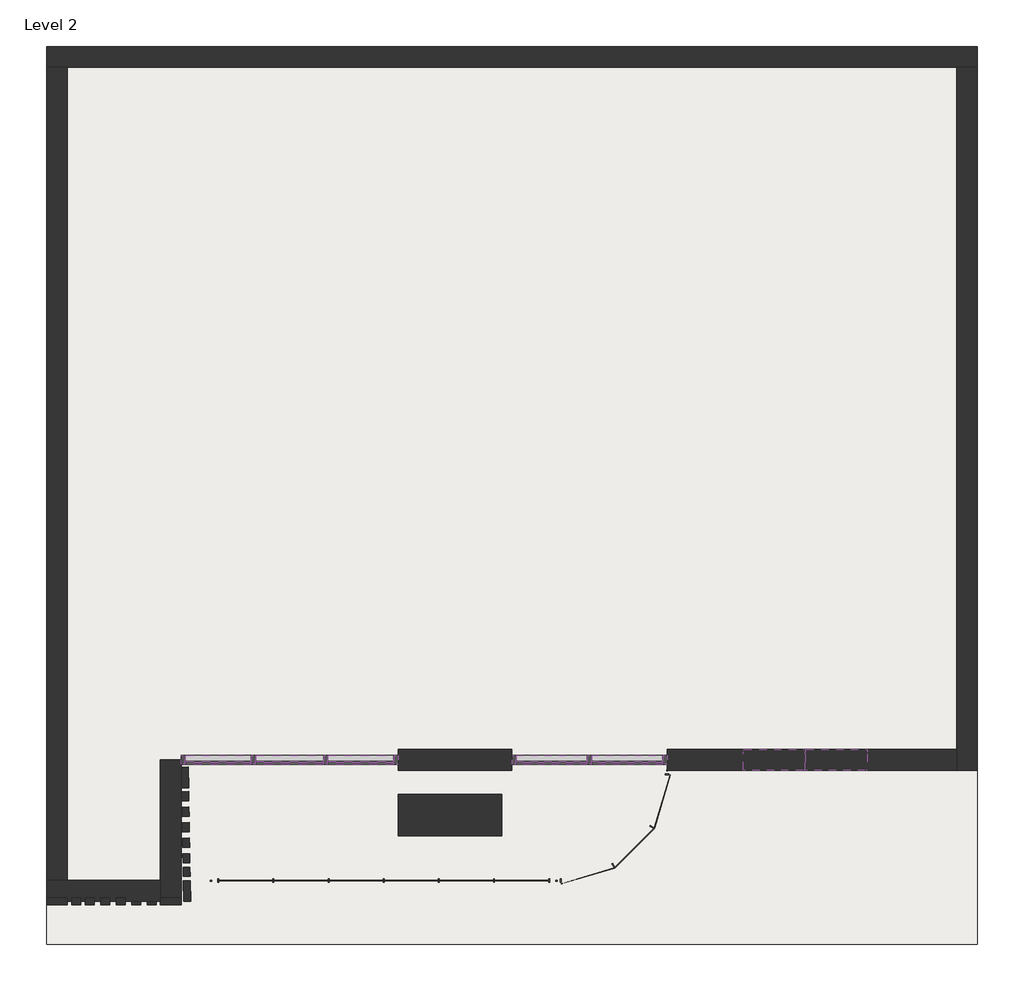
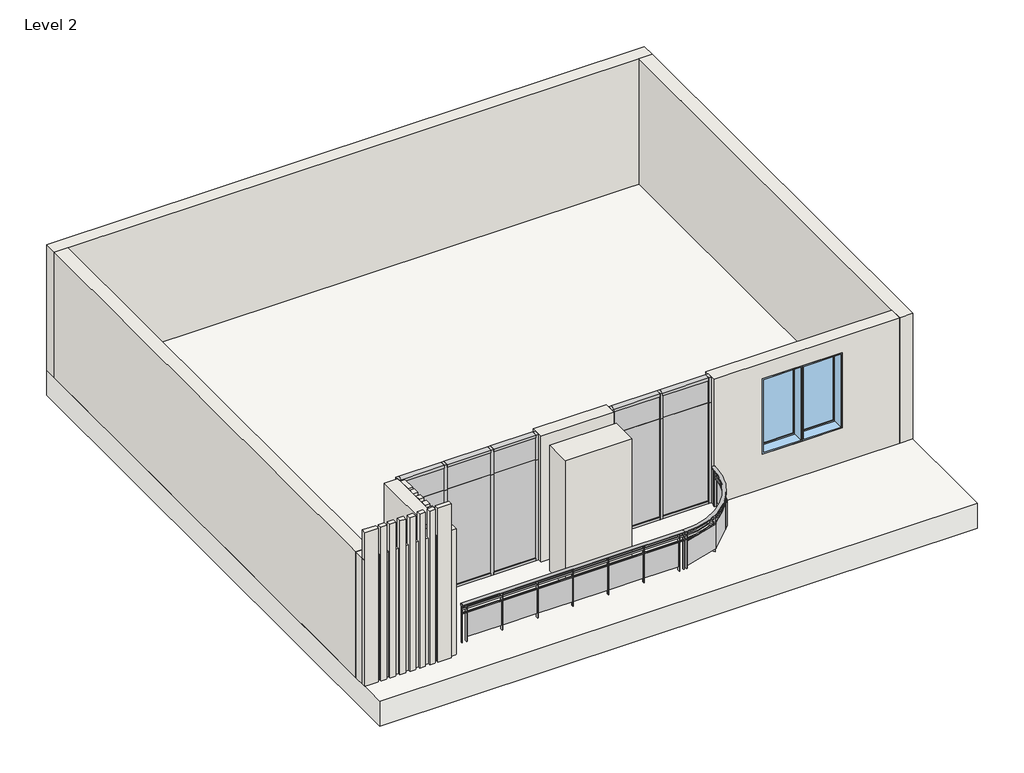
# One storey: 24 members, 24 walls, 10 plates, 2 windows, 1 railing, 1 roof.
"""IFC4 building model written with IfcOpenShell, lengths in millimetres."""

from ifc_helpers import new_model, si_unit, point, frame, origin, place, context, project, spatial, polyline, circle_curve, ellipse_curve, trimmed, outline, extrude, faceted_brep, transform, mapped, element, save
from ifc_brep_helpers import plane_surface, cylinder_surface, revolved_surface, extruded_surface, advanced_brep
from components import member_78934672, member_801a2072, member_cfcad22e, member_ee409385, member_47bfaf8a, member_f0fea5a5, member_6e77e263, system_panel_glazed_66ef8e2c, system_panel_glazed_30b75583, system_panel_glazed_387c9df4, system_panel_glazed_55a8196a, system_panel_glazed_9df4f396, system_panel_glazed_c1629c18, window_9a1f8bc2, window_c524ad49

model = new_model("IFC4")

# Units and contexts
model_context = context("Model", 3, world=origin())
ifc_project = project(units=[si_unit("LENGTHUNIT", "METRE", prefix="MILLI")], contexts=[model_context])

# Site, building, storey
site = spatial("IfcSite", under=ifc_project)
building = spatial("IfcBuilding", under=site)
storey = spatial("IfcBuildingStorey", under=building, Name="Level 2", Elevation=3048.0)

# Members
placement = place(None, origin())
member_shape = member_78934672(model_context)
element("IfcMember", 1, ObjectType="Rectangular Mullion : 2.5\" x 5\" rectangular", at=placement, inside=storey, context=model_context, shape_type="MappedRepresentation", body=[
    mapped(member_shape, transform((-10103.7104559, 977.728737, 3657.6), x_axis=(0.0, 0.0, -1.0), y_axis=(0.0, 1.0, 0.0), z_axis=(1.0, 0.0, 0.0))),
])
element("IfcMember", 2, ObjectType="Rectangular Mullion : 2.5\" x 5\" rectangular", at=placement, inside=storey, context=model_context, shape_type="MappedRepresentation", body=[
    mapped(member_shape, transform((-11214.9604559, 977.728737, 3657.6), x_axis=(0.0, 0.0, -1.0), y_axis=(0.0, 1.0, 0.0), z_axis=(1.0, 0.0, 0.0))),
])
element("IfcMember", 3, ObjectType="Rectangular Mullion : 2.5\" x 5\" rectangular", at=placement, inside=storey, context=model_context, shape_type="MappedRepresentation", body=[
    mapped(member_shape, transform((-12262.7104559, 977.728737, 6705.6), x_axis=(0.0, 0.0, 1.0), y_axis=(0.0, 1.0, 0.0), z_axis=(-1.0, 0.0, 0.0))),
])
element("IfcMember", 4, ObjectType="Rectangular Mullion : 2.5\" x 5\" rectangular", at=placement, inside=storey, context=model_context, shape_type="MappedRepresentation", body=[
    mapped(member_shape, transform((-11151.4604559, 977.728737, 6705.6), x_axis=(0.0, 0.0, 1.0), y_axis=(0.0, 1.0, 0.0), z_axis=(-1.0, 0.0, 0.0))),
])
member_2_shape = member_801a2072(model_context)
element("IfcMember", 5, ObjectType="Rectangular Mullion : 2.5\" x 5\" rectangular", at=placement, inside=storey, context=model_context, shape_type="MappedRepresentation", body=[
    mapped(member_2_shape, transform((-17139.5104559, 977.728737, 6705.6), x_axis=(0.0, 0.0, 1.0), y_axis=(0.0, 1.0, 0.0), z_axis=(-1.0, 0.0, 0.0))),
])
element("IfcMember", 6, ObjectType="Rectangular Mullion : 2.5\" x 5\" rectangular", at=placement, inside=storey, context=model_context, shape_type="MappedRepresentation", body=[
    mapped(member_2_shape, transform((-15037.6604559, 977.728737, 6705.6), x_axis=(0.0, 0.0, 1.0), y_axis=(0.0, 1.0, 0.0), z_axis=(-1.0, 0.0, 0.0))),
])
element("IfcMember", 7, ObjectType="Rectangular Mullion : 2.5\" x 5\" rectangular", at=placement, inside=storey, context=model_context, shape_type="MappedRepresentation", body=[
    mapped(member_2_shape, transform((-14066.1104559, 977.728737, 3657.6), x_axis=(0.0, 0.0, -1.0), y_axis=(0.0, 1.0, 0.0), z_axis=(1.0, 0.0, 0.0))),
])
element("IfcMember", 8, ObjectType="Rectangular Mullion : 2.5\" x 5\" rectangular", at=placement, inside=storey, context=model_context, shape_type="MappedRepresentation", body=[
    mapped(member_2_shape, transform((-16167.9604559, 977.728737, 3657.6), x_axis=(0.0, 0.0, -1.0), y_axis=(0.0, 1.0, 0.0), z_axis=(1.0, 0.0, 0.0))),
])
member_3_shape = member_cfcad22e(model_context)
element("IfcMember", 9, ObjectType="Rectangular Mullion : 2.5\" x 5\" rectangular", at=placement, inside=storey, context=model_context, shape_type="MappedRepresentation", body=[
    mapped(member_3_shape, transform((-15101.1604559, 977.728737, 3657.6), x_axis=(0.0, 0.0, -1.0), y_axis=(0.0, 1.0, 0.0), z_axis=(1.0, 0.0, 0.0))),
])
element("IfcMember", 10, ObjectType="Rectangular Mullion : 2.5\" x 5\" rectangular", at=placement, inside=storey, context=model_context, shape_type="MappedRepresentation", body=[
    mapped(member_3_shape, transform((-16104.4604559, 977.728737, 6705.6), x_axis=(0.0, 0.0, 1.0), y_axis=(0.0, 1.0, 0.0), z_axis=(-1.0, 0.0, 0.0))),
])
member_4_shape = member_ee409385(model_context)
element("IfcMember", 11, ObjectType="Rectangular Mullion : 2.5\" x 5\" rectangular", at=placement, inside=storey, context=model_context, shape_type="MappedRepresentation", body=[
    mapped(member_4_shape, transform((-12326.2104559, 977.728737, 3657.6), x_axis=(-1.0, 0.0, 0.0), y_axis=(0.0, 1.0, 0.0), z_axis=(0.0, 0.0, -1.0))),
])
element("IfcMember", 12, ObjectType="Rectangular Mullion : 2.5\" x 5\" rectangular", at=placement, inside=storey, context=model_context, shape_type="MappedRepresentation", body=[
    mapped(member_4_shape, transform((-17203.0104559, 977.728737, 3657.6), x_axis=(-1.0, 0.0, 0.0), y_axis=(0.0, 1.0, 0.0), z_axis=(0.0, 0.0, -1.0))),
])
member_5_shape = member_47bfaf8a(model_context)
element("IfcMember", 13, ObjectType="Rectangular Mullion : 2.5\" x 5\" rectangular", at=placement, inside=storey, context=model_context, shape_type="MappedRepresentation", body=[
    mapped(member_5_shape, transform((-12326.2104559, 977.728737, 6096.0), x_axis=(-1.0, 0.0, 0.0), y_axis=(0.0, 1.0, 0.0), z_axis=(0.0, 0.0, -1.0))),
])
element("IfcMember", 14, ObjectType="Rectangular Mullion : 2.5\" x 5\" rectangular", at=placement, inside=storey, context=model_context, shape_type="MappedRepresentation", body=[
    mapped(member_5_shape, transform((-17203.0104559, 977.728737, 6096.0), x_axis=(-1.0, 0.0, 0.0), y_axis=(0.0, 1.0, 0.0), z_axis=(0.0, 0.0, -1.0))),
])
member_6_shape = member_f0fea5a5(model_context)
element("IfcMember", 15, ObjectType="Rectangular Mullion : 2.5\" x 5\" rectangular", at=placement, inside=storey, context=model_context, shape_type="MappedRepresentation", body=[
    mapped(member_6_shape, transform((-11183.2104559, 977.728737, 3657.6), x_axis=(-1.0, 0.0, 0.0), y_axis=(0.0, 1.0, 0.0), z_axis=(0.0, 0.0, -1.0))),
])
element("IfcMember", 16, ObjectType="Rectangular Mullion : 2.5\" x 5\" rectangular", at=placement, inside=storey, context=model_context, shape_type="MappedRepresentation", body=[
    mapped(member_6_shape, transform((-15069.4104559, 977.728737, 3657.6), x_axis=(-1.0, 0.0, 0.0), y_axis=(0.0, 1.0, 0.0), z_axis=(0.0, 0.0, -1.0))),
])
element("IfcMember", 17, ObjectType="Rectangular Mullion : 2.5\" x 5\" rectangular", at=placement, inside=storey, context=model_context, shape_type="MappedRepresentation", body=[
    mapped(member_6_shape, transform((-16136.2104559, 977.728737, 3657.6), x_axis=(-1.0, 0.0, 0.0), y_axis=(0.0, 1.0, 0.0), z_axis=(0.0, 0.0, -1.0))),
])
member_7_shape = member_6e77e263(model_context)
element("IfcMember", 18, ObjectType="Rectangular Mullion : 2.5\" x 5\" rectangular", at=placement, inside=storey, context=model_context, shape_type="MappedRepresentation", body=[
    mapped(member_7_shape, transform((-11183.2104559, 977.728737, 6096.0), x_axis=(-1.0, 0.0, 0.0), y_axis=(0.0, 1.0, 0.0), z_axis=(0.0, 0.0, -1.0))),
])
element("IfcMember", 19, ObjectType="Rectangular Mullion : 2.5\" x 5\" rectangular", at=placement, inside=storey, context=model_context, shape_type="MappedRepresentation", body=[
    mapped(member_7_shape, transform((-15069.4104559, 977.728737, 6096.0), x_axis=(-1.0, 0.0, 0.0), y_axis=(0.0, 1.0, 0.0), z_axis=(0.0, 0.0, -1.0))),
])
element("IfcMember", 20, ObjectType="Rectangular Mullion : 2.5\" x 5\" rectangular", at=placement, inside=storey, context=model_context, shape_type="MappedRepresentation", body=[
    mapped(member_7_shape, transform((-16136.2104559, 977.728737, 6096.0), x_axis=(-1.0, 0.0, 0.0), y_axis=(0.0, 1.0, 0.0), z_axis=(0.0, 0.0, -1.0))),
])
element("IfcMember", 21, ObjectType="Rectangular Mullion : 2.5\" x 5\" rectangular", at=placement, inside=storey, context=model_context, shape_type="MappedRepresentation", body=[
    mapped(member_5_shape, transform((-10040.2104559, 977.728737, 6705.6), x_axis=(1.0, 0.0, 0.0), y_axis=(0.0, 1.0, 0.0), z_axis=(0.0, 0.0, 1.0))),
])
element("IfcMember", 22, ObjectType="Rectangular Mullion : 2.5\" x 5\" rectangular", at=placement, inside=storey, context=model_context, shape_type="MappedRepresentation", body=[
    mapped(member_5_shape, transform((-14002.6104559, 977.728737, 6705.6), x_axis=(1.0, 0.0, 0.0), y_axis=(0.0, 1.0, 0.0), z_axis=(0.0, 0.0, 1.0))),
])
element("IfcMember", 23, ObjectType="Rectangular Mullion : 2.5\" x 5\" rectangular", at=placement, inside=storey, context=model_context, shape_type="MappedRepresentation", body=[
    mapped(member_4_shape, transform((-10040.2104559, 977.728737, 6096.0), x_axis=(1.0, 0.0, 0.0), y_axis=(0.0, 1.0, 0.0), z_axis=(0.0, 0.0, 1.0))),
])
element("IfcMember", 24, ObjectType="Rectangular Mullion : 2.5\" x 5\" rectangular", at=placement, inside=storey, context=model_context, shape_type="MappedRepresentation", body=[
    mapped(member_4_shape, transform((-14002.6104559, 977.728737, 6096.0), x_axis=(1.0, 0.0, 0.0), y_axis=(0.0, 1.0, 0.0), z_axis=(0.0, 0.0, 1.0))),
])

# Plates
system_panel_glazed_shape = system_panel_glazed_66ef8e2c(model_context)
element("IfcPlate", 25, ObjectType="System Panel : Glazed", at=placement, inside=storey, context=model_context, shape_type="MappedRepresentation", body=[
    mapped(system_panel_glazed_shape, transform((-10627.5854559, 977.728737, 3721.1), x_axis=(-1.0, 0.0, 0.0), y_axis=(0.0, -1.0, 0.0), z_axis=(0.0, 0.0, 1.0))),
])
element("IfcPlate", 26, ObjectType="System Panel : Glazed", at=placement, inside=storey, context=model_context, shape_type="MappedRepresentation", body=[
    mapped(system_panel_glazed_shape, transform((-11738.8354559, 977.728737, 3721.1), x_axis=(-1.0, 0.0, 0.0), y_axis=(0.0, -1.0, 0.0), z_axis=(0.0, 0.0, 1.0))),
])
system_panel_glazed_2_shape = system_panel_glazed_30b75583(model_context)
element("IfcPlate", 27, ObjectType="System Panel : Glazed", at=placement, inside=storey, context=model_context, shape_type="MappedRepresentation", body=[
    mapped(system_panel_glazed_2_shape, transform((-10627.5854559, 977.728737, 6096.0), x_axis=(-1.0, 0.0, 0.0), y_axis=(0.0, -1.0, 0.0), z_axis=(0.0, 0.0, 1.0))),
])
element("IfcPlate", 28, ObjectType="System Panel : Glazed", at=placement, inside=storey, context=model_context, shape_type="MappedRepresentation", body=[
    mapped(system_panel_glazed_2_shape, transform((-11738.8354559, 977.728737, 6096.0), x_axis=(-1.0, 0.0, 0.0), y_axis=(0.0, -1.0, 0.0), z_axis=(0.0, 0.0, 1.0))),
])
system_panel_glazed_3_shape = system_panel_glazed_387c9df4(model_context)
element("IfcPlate", 29, ObjectType="System Panel : Glazed", at=placement, inside=storey, context=model_context, shape_type="MappedRepresentation", body=[
    mapped(system_panel_glazed_3_shape, transform((-14551.8854559, 977.728737, 3721.1), x_axis=(-1.0, 0.0, 0.0), y_axis=(0.0, -1.0, 0.0), z_axis=(0.0, 0.0, 1.0))),
])
element("IfcPlate", 30, ObjectType="System Panel : Glazed", at=placement, inside=storey, context=model_context, shape_type="MappedRepresentation", body=[
    mapped(system_panel_glazed_3_shape, transform((-16653.7354559, 977.728737, 3721.1), x_axis=(-1.0, 0.0, 0.0), y_axis=(0.0, -1.0, 0.0), z_axis=(0.0, 0.0, 1.0))),
])
system_panel_glazed_4_shape = system_panel_glazed_55a8196a(model_context)
element("IfcPlate", 31, ObjectType="System Panel : Glazed", at=placement, inside=storey, context=model_context, shape_type="MappedRepresentation", body=[
    mapped(system_panel_glazed_4_shape, transform((-14551.8854559, 977.728737, 6096.0), x_axis=(-1.0, 0.0, 0.0), y_axis=(0.0, -1.0, 0.0), z_axis=(0.0, 0.0, 1.0))),
])
element("IfcPlate", 32, ObjectType="System Panel : Glazed", at=placement, inside=storey, context=model_context, shape_type="MappedRepresentation", body=[
    mapped(system_panel_glazed_4_shape, transform((-16653.7354559, 977.728737, 6096.0), x_axis=(-1.0, 0.0, 0.0), y_axis=(0.0, -1.0, 0.0), z_axis=(0.0, 0.0, 1.0))),
])
system_panel_glazed_5_shape = system_panel_glazed_9df4f396(model_context)
element("IfcPlate", 33, ObjectType="System Panel : Glazed", at=placement, inside=storey, context=model_context, shape_type="MappedRepresentation", body=[
    mapped(system_panel_glazed_5_shape, transform((-15602.8104559, 977.728737, 3721.1), x_axis=(-1.0, 0.0, 0.0), y_axis=(0.0, -1.0, 0.0), z_axis=(0.0, 0.0, 1.0))),
])
system_panel_glazed_6_shape = system_panel_glazed_c1629c18(model_context)
element("IfcPlate", 34, ObjectType="System Panel : Glazed", at=placement, inside=storey, context=model_context, shape_type="MappedRepresentation", body=[
    mapped(system_panel_glazed_6_shape, transform((-15602.8104559, 977.728737, 6096.0), x_axis=(-1.0, 0.0, 0.0), y_axis=(0.0, -1.0, 0.0), z_axis=(0.0, 0.0, 1.0))),
])

# Railing
element("IfcRailing", 35, ObjectType="Glass Panel - Bottom Fill", at=placement, inside=storey, context=model_context, shape_type="SolidModel", body=[
    advanced_brep(
    [(-16762.7787181, -765.7171954, 4572.0), (-16762.7787181, -841.9171954, 4572.0), (-11669.3563882, -765.7171954, 4572.0), (-11669.3563882, -841.9171954, 4572.0), (-10002.1104559, 825.328737, 4572.0), (-10078.3104559, 825.328737, 4572.0)],
    [
        (0, 1, ellipse_curve(frame((-16762.7787181, -803.8171954, 4572.0), z_axis=(-1.0, 0.0, 0.0), x_axis=(0.0, -1.0, 0.0)), 38.1, 28.575)),
        (1, 0, ellipse_curve(frame((-16762.7787181, -803.8171954, 4572.0), z_axis=(-1.0, 0.0, 0.0), x_axis=(0.0, -1.0, 0.0)), 38.1, 28.575)),
        (0, 2),
        (2, 3, ellipse_curve(frame((-11669.3563882, -803.8171954, 4572.0), z_axis=(-1.0, 0.0, 0.0), x_axis=(0.0, -1.0, 0.0)), 38.1, 28.575)),
        (3, 1),
        (3, 2, ellipse_curve(frame((-11669.3563882, -803.8171954, 4572.0), z_axis=(-1.0, 0.0, 0.0), x_axis=(0.0, -1.0, 0.0)), 38.1, 28.575)),
        (4, 3, circle_curve(frame((-11669.3563882, 825.328737, 4572.0), z_axis=(0.0, 0.0, -1.0), x_axis=(0.0, -1.0, 0.0)), 1667.2459324)),
        (2, 5, circle_curve(frame((-11669.3563882, 825.328737, 4572.0), z_axis=(0.0, 0.0, 1.0), x_axis=(0.0, -1.0, 0.0)), 1591.0459324)),
        (5, 4, ellipse_curve(frame((-10040.2104559, 825.328737, 4572.0), z_axis=(0.0, -1.0, 0.0), x_axis=(1.0, 0.0, 0.0)), 38.1, 28.575)),
        (4, 5, ellipse_curve(frame((-10040.2104559, 825.328737, 4572.0), z_axis=(0.0, -1.0, 0.0), x_axis=(1.0, 0.0, 0.0)), 38.1, 28.575)),
    ],
    [
        plane_surface(frame((-16762.7787181, -803.8171954, 4572.0), z_axis=(-1.0, 0.0, 0.0), x_axis=(0.0, 1.0, 0.0))),
        extruded_surface(trimmed(ellipse_curve(frame((-11669.3563882, -803.8171954, 4572.0), z_axis=(-1.0, 0.0, 0.0), x_axis=(0.0, -1.0, 0.0)), 38.1, 28.575), [point((-11669.3563882, -765.7171954, 4572.0))], [point((-11669.3563882, -841.9171954, 4572.0))], True, "CARTESIAN"), (-5093.422329899999, 0.0, 0.0), 5093.422329899999),
        extruded_surface(trimmed(ellipse_curve(frame((-11669.3563882, -803.8171954, 4572.0), z_axis=(-1.0, 0.0, 0.0), x_axis=(0.0, -1.0, 0.0)), 38.1, 28.575), [point((-11669.3563882, -841.9171954, 4572.0))], [point((-11669.3563882, -765.7171954, 4572.0))], True, "CARTESIAN"), (-5093.422329899999, 0.0, 0.0), 5093.422329899999),
        revolved_surface(trimmed(ellipse_curve(frame((-11669.3563882, -803.8171954, 4572.0), z_axis=(-1.0, 0.0, 0.0), x_axis=(0.0, -1.0, 0.0)), 38.1, 28.575), [point((-11669.3563882, -765.7171954, 4572.0))], [point((-11669.3563882, -841.9171954, 4572.0))], True, "CARTESIAN"), (-11669.3563882, 825.328737, 4572.0), (0.0, 0.0, 1.0)),
        revolved_surface(trimmed(ellipse_curve(frame((-11669.3563882, -803.8171954, 4572.0), z_axis=(-1.0, 0.0, 0.0), x_axis=(0.0, -1.0, 0.0)), 38.1, 28.575), [point((-11669.3563882, -841.9171954, 4572.0))], [point((-11669.3563882, -765.7171954, 4572.0))], True, "CARTESIAN"), (-11669.3563882, 825.328737, 4572.0), (0.0, 0.0, 1.0)),
        plane_surface(frame((-10040.2104559, 825.328737, 4572.0), z_axis=(0.0, 1.0, 0.0), x_axis=(0.0, 0.0, 1.0))),
    ],
    [
        (0, [[1, 2]]),
        (1, [[-1, 3, 4, 5]]),
        (2, [[-2, -5, 6, -3]]),
        (3, [[7, -4, 8, 9]]),
        (4, [[-8, -6, -7, 10]]),
        (5, [[-10, -9]]),
    ],
),
    advanced_brep(
    [(-16762.7787181, -816.5171954, 4483.1), (-16762.7787181, -791.1171954, 4483.1), (-16762.7787181, -791.1171954, 4457.7), (-16762.7787181, -816.5171954, 4457.7), (-11669.3563882, -816.5171954, 4483.1), (-11669.3563882, -791.1171954, 4483.1), (-11669.3563882, -791.1171954, 4457.7), (-11669.3563882, -816.5171954, 4457.7), (-10052.9104559, 825.328737, 4483.1), (-10027.5104559, 825.328737, 4483.1), (-10052.9104559, 825.328737, 4457.7), (-10027.5104559, 825.328737, 4457.7)],
    [
        (0, 1),
        (1, 2),
        (2, 3),
        (3, 0),
        (0, 4),
        (4, 5),
        (5, 1),
        (5, 6),
        (6, 2),
        (6, 7),
        (7, 3),
        (7, 4),
        (8, 5, circle_curve(frame((-11669.3563882, 825.328737, 4483.1), z_axis=(0.0, 0.0, -1.0), x_axis=(0.0, -1.0, 0.0)), 1616.4459324)),
        (4, 9, circle_curve(frame((-11669.3563882, 825.328737, 4483.1), z_axis=(0.0, 0.0, 1.0), x_axis=(0.0, -1.0, 0.0)), 1641.8459324)),
        (9, 8),
        (10, 6, circle_curve(frame((-11669.3563882, 825.328737, 4457.7), z_axis=(0.0, 0.0, -1.0), x_axis=(0.0, -1.0, 0.0)), 1616.4459324)),
        (8, 10),
        (11, 7, circle_curve(frame((-11669.3563882, 825.328737, 4457.7), z_axis=(0.0, 0.0, -1.0), x_axis=(0.0, -1.0, 0.0)), 1641.8459324)),
        (10, 11),
        (11, 9),
    ],
    [
        plane_surface(frame((-16762.7787181, -803.8171954, 4470.4), z_axis=(-1.0, 0.0, 0.0), x_axis=(0.0, 1.0, 0.0))),
        plane_surface(frame((-16762.7787181, -816.5171954, 4483.1), z_axis=(0.0, 0.0, 1.0), x_axis=(1.0, 0.0, 0.0))),
        plane_surface(frame((-16762.7787181, -791.1171954, 4483.1), z_axis=(0.0, 1.0, 0.0), x_axis=(1.0, 0.0, 0.0))),
        plane_surface(frame((-16762.7787181, -791.1171954, 4457.7), z_axis=(0.0, 0.0, -1.0), x_axis=(1.0, 0.0, 0.0))),
        plane_surface(frame((-16762.7787181, -816.5171954, 4457.7), z_axis=(0.0, -1.0, 0.0), x_axis=(1.0, 0.0, 0.0))),
        plane_surface(frame((-11669.3563882, 825.328737, 4483.1), z_axis=(0.0, 0.0, 1.0), x_axis=(0.0, -1.0, 0.0))),
        revolved_surface(polyline([(-11669.3563882, -791.1171953999999, 4483.1), (-11669.3563882, -791.1171953999999, 4457.7)]), (-11669.3563882, 825.328737, 4470.4), (0.0, 0.0, 1.0)),
        plane_surface(frame((-11669.3563882, 825.328737, 4457.7), z_axis=(0.0, 0.0, -1.0), x_axis=(0.0, -1.0, 0.0))),
        cylinder_surface(frame((-11669.3563882, 825.328737, 4470.4), z_axis=(0.0, 0.0, 1.0), x_axis=(0.0, -1.0, 0.0)), 1641.8459324),
        plane_surface(frame((-10040.2104559, 825.328737, 4470.4), z_axis=(0.0, 1.0, 0.0), x_axis=(0.0, 0.0, 1.0))),
    ],
    [
        (0, [[1, 2, 3, 4]]),
        (1, [[-1, 5, 6, 7]]),
        (2, [[-2, -7, 8, 9]]),
        (3, [[-3, -9, 10, 11]]),
        (4, [[-4, -11, 12, -5]]),
        (5, [[13, -6, 14, 15]]),
        (6, [[16, -8, -13, 17]]),
        (7, [[18, -10, -16, 19]]),
        (8, [[-14, -12, -18, 20]]),
        (9, [[-20, -19, -17, -15]]),
    ],
),
    advanced_brep(
    [(-16762.7787181, -816.5171954, 4381.5), (-16762.7787181, -791.1171954, 4381.5), (-16762.7787181, -791.1171954, 4356.1), (-16762.7787181, -816.5171954, 4356.1), (-11669.3563882, -816.5171954, 4381.5), (-11669.3563882, -791.1171954, 4381.5), (-11669.3563882, -791.1171954, 4356.1), (-11669.3563882, -816.5171954, 4356.1), (-10052.9104559, 825.328737, 4381.5), (-10027.5104559, 825.328737, 4381.5), (-10052.9104559, 825.328737, 4356.1), (-10027.5104559, 825.328737, 4356.1)],
    [
        (0, 1),
        (1, 2),
        (2, 3),
        (3, 0),
        (0, 4),
        (4, 5),
        (5, 1),
        (5, 6),
        (6, 2),
        (6, 7),
        (7, 3),
        (7, 4),
        (8, 5, circle_curve(frame((-11669.3563882, 825.328737, 4381.5), z_axis=(0.0, 0.0, -1.0), x_axis=(0.0, -1.0, 0.0)), 1616.4459324)),
        (4, 9, circle_curve(frame((-11669.3563882, 825.328737, 4381.5), z_axis=(0.0, 0.0, 1.0), x_axis=(0.0, -1.0, 0.0)), 1641.8459324)),
        (9, 8),
        (10, 6, circle_curve(frame((-11669.3563882, 825.328737, 4356.1), z_axis=(0.0, 0.0, -1.0), x_axis=(0.0, -1.0, 0.0)), 1616.4459324)),
        (8, 10),
        (11, 7, circle_curve(frame((-11669.3563882, 825.328737, 4356.1), z_axis=(0.0, 0.0, -1.0), x_axis=(0.0, -1.0, 0.0)), 1641.8459324)),
        (10, 11),
        (11, 9),
    ],
    [
        plane_surface(frame((-16762.7787181, -803.8171954, 4368.8), z_axis=(-1.0, 0.0, 0.0), x_axis=(0.0, 1.0, 0.0))),
        plane_surface(frame((-16762.7787181, -816.5171954, 4381.5), z_axis=(0.0, 0.0, 1.0), x_axis=(1.0, 0.0, 0.0))),
        plane_surface(frame((-16762.7787181, -791.1171954, 4381.5), z_axis=(0.0, 1.0, 0.0), x_axis=(1.0, 0.0, 0.0))),
        plane_surface(frame((-16762.7787181, -791.1171954, 4356.1), z_axis=(0.0, 0.0, -1.0), x_axis=(1.0, 0.0, 0.0))),
        plane_surface(frame((-16762.7787181, -816.5171954, 4356.1), z_axis=(0.0, -1.0, 0.0), x_axis=(1.0, 0.0, 0.0))),
        plane_surface(frame((-11669.3563882, 825.328737, 4381.5), z_axis=(0.0, 0.0, 1.0), x_axis=(0.0, -1.0, 0.0))),
        revolved_surface(polyline([(-11669.3563882, -791.1171953999999, 4381.5), (-11669.3563882, -791.1171953999999, 4356.1)]), (-11669.3563882, 825.328737, 4368.8), (0.0, 0.0, 1.0)),
        plane_surface(frame((-11669.3563882, 825.328737, 4356.1), z_axis=(0.0, 0.0, -1.0), x_axis=(0.0, -1.0, 0.0))),
        cylinder_surface(frame((-11669.3563882, 825.328737, 4368.8), z_axis=(0.0, 0.0, 1.0), x_axis=(0.0, -1.0, 0.0)), 1641.8459324),
        plane_surface(frame((-10040.2104559, 825.328737, 4368.8), z_axis=(0.0, 1.0, 0.0), x_axis=(0.0, 0.0, 1.0))),
    ],
    [
        (0, [[1, 2, 3, 4]]),
        (1, [[-1, 5, 6, 7]]),
        (2, [[-2, -7, 8, 9]]),
        (3, [[-3, -9, 10, 11]]),
        (4, [[-4, -11, 12, -5]]),
        (5, [[13, -6, 14, 15]]),
        (6, [[16, -8, -13, 17]]),
        (7, [[18, -10, -16, 19]]),
        (8, [[-14, -12, -18, 20]]),
        (9, [[-20, -19, -17, -15]]),
    ],
),
    extrude(outline(polyline([(-10016.1798264, 757.7282919), (-10066.9450003, 759.6090156), (-10066.4748193, 772.3003091), (-10015.7096455, 770.4195853), (-10016.1798264, 757.7282919)])), frame((0.0, 0.0, 3657.6), z_axis=(0.0, 0.0, 1.0), x_axis=(1.0, 0.0, 0.0)), (0.0, 0.0, 1.0), 885.6788223),
    extrude(outline(polyline([(-10227.7208829, -23.0307141), (-9998.0369146, 756.6417265), (-9991.9457237, 754.8473205), (-10221.629692, -24.8251201), (-10227.7208829, -23.0307141)])), frame((0.0, 0.0, 3759.2), z_axis=(0.0, 0.0, 1.0), x_axis=(1.0, 0.0, 0.0)), (0.0, 0.0, 1.0), 596.9),
    extrude(outline(polyline([(-10250.0405804, -25.0271899), (-10293.7178017, 0.9139036), (-10287.2325284, 11.8332089), (-10243.555307, -14.1078846), (-10250.0405804, -25.0271899)])), frame((0.0, 0.0, 3657.6), z_axis=(0.0, 0.0, 1.0), x_axis=(1.0, 0.0, 0.0)), (0.0, 0.0, 1.0), 885.6788223),
    extrude(outline(polyline([(-10809.3655016, -609.3985414), (-10234.6291099, -34.6621497), (-10230.1389818, -39.1522777), (-10804.8753736, -613.8886695), (-10809.3655016, -609.3985414)])), frame((0.0, 0.0, 3759.2), z_axis=(0.0, 0.0, 1.0), x_axis=(1.0, 0.0, 0.0)), (0.0, 0.0, 1.0), 596.9),
    extrude(outline(polyline([(-10829.9197667, -600.4723443), (-10855.8608602, -556.7951229), (-10844.9415549, -550.3098495), (-10819.0004614, -593.9870709), (-10829.9197667, -600.4723443)])), frame((0.0, 0.0, 3657.6), z_axis=(0.0, 0.0, 1.0), x_axis=(1.0, 0.0, 0.0)), (0.0, 0.0, 1.0), 885.6788223),
    extrude(outline(polyline([(-11600.6693778, -845.9907367), (-10820.9969372, -616.3067684), (-10819.2025312, -622.3979593), (-11598.8749718, -852.0819276), (-11600.6693778, -845.9907367)])), frame((0.0, 0.0, 3759.2), z_axis=(0.0, 0.0, 1.0), x_axis=(1.0, 0.0, 0.0)), (0.0, 0.0, 1.0), 596.9),
    extrude(outline(polyline([(-11614.4472366, -828.3180058), (-11616.3279603, -777.552832), (-11603.6366669, -777.082651), (-11601.7559432, -827.8478249), (-11614.4472366, -828.3180058)])), frame((0.0, 0.0, 3657.6), z_axis=(0.0, 0.0, 1.0), x_axis=(1.0, 0.0, 0.0)), (0.0, 0.0, 1.0), 885.6788223),
    extrude(outline(polyline([(-11784.0175532, -829.2171954), (-11784.0175532, -778.4171954), (-11771.3175532, -778.4171954), (-11771.3175532, -829.2171954), (-11784.0175532, -829.2171954)])), frame((0.0, 0.0, 3657.6), z_axis=(0.0, 0.0, 1.0), x_axis=(1.0, 0.0, 0.0)), (0.0, 0.0, 1.0), 885.6788223),
    extrude(outline(polyline([(-12590.4675532, -797.2820384), (-11777.6675532, -797.2820384), (-11777.6675532, -803.6320384), (-12590.4675532, -803.6320384), (-12590.4675532, -797.2820384)])), frame((0.0, 0.0, 3759.2), z_axis=(0.0, 0.0, 1.0), x_axis=(1.0, 0.0, 0.0)), (0.0, 0.0, 1.0), 596.9),
    extrude(outline(polyline([(-12596.8175532, -829.2171954), (-12596.8175532, -778.4171954), (-12584.1175532, -778.4171954), (-12584.1175532, -829.2171954), (-12596.8175532, -829.2171954)])), frame((0.0, 0.0, 3657.6), z_axis=(0.0, 0.0, 1.0), x_axis=(1.0, 0.0, 0.0)), (0.0, 0.0, 1.0), 885.6788223),
    extrude(outline(polyline([(-13403.2675532, -797.2820384), (-12590.4675532, -797.2820384), (-12590.4675532, -803.6320384), (-13403.2675532, -803.6320384), (-13403.2675532, -797.2820384)])), frame((0.0, 0.0, 3759.2), z_axis=(0.0, 0.0, 1.0), x_axis=(1.0, 0.0, 0.0)), (0.0, 0.0, 1.0), 596.9),
    extrude(outline(polyline([(-13409.6175532, -829.2171954), (-13409.6175532, -778.4171954), (-13396.9175532, -778.4171954), (-13396.9175532, -829.2171954), (-13409.6175532, -829.2171954)])), frame((0.0, 0.0, 3657.6), z_axis=(0.0, 0.0, 1.0), x_axis=(1.0, 0.0, 0.0)), (0.0, 0.0, 1.0), 885.6788223),
    extrude(outline(polyline([(-14216.0675532, -797.2820384), (-13403.2675532, -797.2820384), (-13403.2675532, -803.6320384), (-14216.0675532, -803.6320384), (-14216.0675532, -797.2820384)])), frame((0.0, 0.0, 3759.2), z_axis=(0.0, 0.0, 1.0), x_axis=(1.0, 0.0, 0.0)), (0.0, 0.0, 1.0), 596.9),
    extrude(outline(polyline([(-14222.4175532, -829.2171954), (-14222.4175532, -778.4171954), (-14209.7175532, -778.4171954), (-14209.7175532, -829.2171954), (-14222.4175532, -829.2171954)])), frame((0.0, 0.0, 3657.6), z_axis=(0.0, 0.0, 1.0), x_axis=(1.0, 0.0, 0.0)), (0.0, 0.0, 1.0), 885.6788223),
    extrude(outline(polyline([(-15028.8675532, -797.2820384), (-14216.0675532, -797.2820384), (-14216.0675532, -803.6320384), (-15028.8675532, -803.6320384), (-15028.8675532, -797.2820384)])), frame((0.0, 0.0, 3759.2), z_axis=(0.0, 0.0, 1.0), x_axis=(1.0, 0.0, 0.0)), (0.0, 0.0, 1.0), 596.9),
    extrude(outline(polyline([(-15035.2175532, -829.2171954), (-15035.2175532, -778.4171954), (-15022.5175532, -778.4171954), (-15022.5175532, -829.2171954), (-15035.2175532, -829.2171954)])), frame((0.0, 0.0, 3657.6), z_axis=(0.0, 0.0, 1.0), x_axis=(1.0, 0.0, 0.0)), (0.0, 0.0, 1.0), 885.6788223),
    extrude(outline(polyline([(-15841.6675532, -797.2820384), (-15028.8675532, -797.2820384), (-15028.8675532, -803.6320384), (-15841.6675532, -803.6320384), (-15841.6675532, -797.2820384)])), frame((0.0, 0.0, 3759.2), z_axis=(0.0, 0.0, 1.0), x_axis=(1.0, 0.0, 0.0)), (0.0, 0.0, 1.0), 596.9),
    extrude(outline(polyline([(-15848.0175532, -829.2171954), (-15848.0175532, -778.4171954), (-15835.3175532, -778.4171954), (-15835.3175532, -829.2171954), (-15848.0175532, -829.2171954)])), frame((0.0, 0.0, 3657.6), z_axis=(0.0, 0.0, 1.0), x_axis=(1.0, 0.0, 0.0)), (0.0, 0.0, 1.0), 885.6788223),
    extrude(outline(polyline([(-16654.4675532, -797.2820384), (-15841.6675532, -797.2820384), (-15841.6675532, -803.6320384), (-16654.4675532, -803.6320384), (-16654.4675532, -797.2820384)])), frame((0.0, 0.0, 3759.2), z_axis=(0.0, 0.0, 1.0), x_axis=(1.0, 0.0, 0.0)), (0.0, 0.0, 1.0), 596.9),
    extrude(outline(polyline([(-16660.8175532, -829.2171954), (-16660.8175532, -778.4171954), (-16648.1175532, -778.4171954), (-16648.1175532, -829.2171954), (-16660.8175532, -829.2171954)])), frame((0.0, 0.0, 3657.6), z_axis=(0.0, 0.0, 1.0), x_axis=(1.0, 0.0, 0.0)), (0.0, 0.0, 1.0), 885.6788223),
    extrude(outline(polyline([(-11678.8813882, -813.3421954), (-11678.8813882, -794.2921954), (-11659.8313882, -794.2921954), (-11659.8313882, -813.3421954), (-11678.8813882, -813.3421954)])), frame((0.0, 0.0, 3657.6), z_axis=(0.0, 0.0, 1.0), x_axis=(1.0, 0.0, 0.0)), (0.0, 0.0, 1.0), 885.6788223),
    extrude(outline(polyline([(-10030.7071308, 812.610194), (-10049.7570946, 812.6473201), (-10049.7199686, 831.6972839), (-10030.6700048, 831.6601579), (-10030.7071308, 812.610194)])), frame((0.0, 0.0, 3657.6), z_axis=(0.0, 0.0, 1.0), x_axis=(1.0, 0.0, 0.0)), (0.0, 0.0, 1.0), 885.6788223),
    extrude(outline(polyline([(-16769.1287181, -813.3421954), (-16769.1287181, -794.2921954), (-16750.0787181, -794.2921954), (-16750.0787181, -813.3421954), (-16769.1287181, -813.3421954)])), frame((0.0, 0.0, 3657.6), z_axis=(0.0, 0.0, 1.0), x_axis=(1.0, 0.0, 0.0)), (0.0, 0.0, 1.0), 885.6788223),
])

# Roof
element("IfcRoof", 36, ObjectType="roof 1", at=placement, inside=storey, context=model_context, shape_type="SweptSolid", body=[
    extrude(outline(polyline([(-19184.2104559, 11493.328737), (-5468.2104559, 11493.328737), (-5468.2104559, -1740.3873511), (-19184.2104559, -1740.3873511), (-19184.2104559, 11493.328737)])), frame((0.0, 0.0, 3048.0), z_axis=(0.0, 0.0, 1.0), x_axis=(1.0, 0.0, 0.0)), (0.0, 0.0, 1.0), 609.6),
])

# Walls
element("IfcWall", 37, ObjectType="Generic - 12\" 2", at=placement, inside=storey, context=model_context, shape_type="Brep", body=[
    faceted_brep([(-19184.2104559, 11188.528737, 3657.6), (-18879.4104559, 11188.528737, 3657.6), (-5773.0104559, 11188.528737, 3657.6), (-5468.2104559, 11188.528737, 3657.6), (-5468.2104559, 11188.528737, 6705.6), (-5773.0104559, 11188.528737, 6705.6), (-18879.4104559, 11188.528737, 6705.6), (-19184.2104559, 11188.528737, 6705.6), (-19184.2104559, 11493.328737, 3657.6), (-19184.2104559, 11493.328737, 6705.6), (-5468.2104559, 11493.328737, 6705.6), (-5468.2104559, 11493.328737, 3657.6)], [[[0, 1, 2, 3, 4, 5, 6, 7]], [[8, 9, 10, 11]], [[3, 2, 1, 0, 8, 11]], [[7, 6, 5, 4, 10, 9]], [[4, 3, 11, 10]], [[0, 7, 9, 8]]]),
])
element("IfcWall", 38, ObjectType="Generic - 12\" 2", at=placement, inside=storey, context=model_context, shape_type="Brep", body=[
    faceted_brep([(-5773.0104559, 11188.528737, 3657.6), (-5773.0104559, 1130.128737, 3657.6), (-5773.0104559, 825.328737, 3657.6), (-5773.0104559, 825.328737, 6705.6), (-5773.0104559, 1130.128737, 6705.6), (-5773.0104559, 11188.528737, 6705.6), (-5468.2104559, 11188.528737, 3657.6), (-5468.2104559, 11188.528737, 6705.6), (-5468.2104559, 825.328737, 6705.6), (-5468.2104559, 825.328737, 3657.6)], [[[0, 1, 2, 3, 4, 5]], [[6, 7, 8, 9]], [[2, 1, 0, 6, 9]], [[5, 4, 3, 8, 7]], [[0, 5, 7, 6]], [[3, 2, 9, 8]]]),
])
element("IfcWall", 39, ObjectType="Generic - 12\" 2", at=placement, inside=storey, context=model_context, shape_type="SweptSolid", body=[
    extrude(outline(polyline([(3657.6, -10040.2104559), (3657.6, -5773.0104559), (6705.6, -5773.0104559), (6705.6, -10040.2104559), (3657.6, -10040.2104559)]), holes=[polyline([(4495.8, -8922.6104559), (6324.6, -8922.6104559), (6324.6, -8008.2104559), (6322.4260244, -8008.2104559), (6322.4260244, -7093.8104559), (4493.6260244, -7093.8104559), (4493.6260244, -8008.2104559), (4495.8, -8008.2104559), (4495.8, -8922.6104559)])]), frame((0.0, 825.328737, 0.0), z_axis=(0.0, 1.0, 0.0), x_axis=(0.0, 0.0, 1.0)), (0.0, 0.0, 1.0), 304.8),
])
element("IfcWall", 40, ObjectType="Generic - 12\" 2", at=placement, inside=storey, context=model_context, shape_type="Brep", body=[
    faceted_brep([(-17507.8104559, 977.728737, 3657.6), (-17507.8104559, -800.271263, 3657.6), (-17507.8104559, -1105.071263, 3657.6), (-17507.8104559, -1105.071263, 6705.6), (-17507.8104559, -800.271263, 6705.6), (-17507.8104559, 977.728737, 6705.6), (-17203.0104559, 977.728737, 3657.6), (-17203.0104559, 977.728737, 6705.6), (-17203.0104559, -1105.071263, 6705.6), (-17203.0104559, -1105.071263, 3657.6)], [[[0, 1, 2, 3, 4, 5]], [[6, 7, 8, 9]], [[2, 1, 0, 6, 9]], [[5, 4, 3, 8, 7]], [[0, 5, 7, 6]], [[3, 2, 9, 8]]]),
])
element("IfcWall", 41, ObjectType="Generic - 12\" 2", at=placement, inside=storey, context=model_context, shape_type="Brep", body=[
    faceted_brep([(-17507.8104559, -800.271263, 3657.6), (-18879.4104559, -800.271263, 3657.6), (-19184.2104559, -800.271263, 3657.6), (-19184.2104559, -800.271263, 6705.6), (-18879.4104559, -800.271263, 6705.6), (-17507.8104559, -800.271263, 6705.6), (-17507.8104559, -1105.071263, 3657.6), (-17507.8104559, -1105.071263, 6705.6), (-19184.2104559, -1105.071263, 6705.6), (-19184.2104559, -1105.071263, 3657.6)], [[[0, 1, 2, 3, 4, 5]], [[6, 7, 8, 9]], [[2, 1, 0, 6, 9]], [[5, 4, 3, 8, 7]], [[0, 5, 7, 6]], [[3, 2, 9, 8]]]),
])
element("IfcWall", 42, ObjectType="Generic - 12\" 2", at=placement, inside=storey, context=model_context, shape_type="SweptSolid", body=[
    extrude(outline(polyline([(-18879.4104559, 11188.528737), (-18879.4104559, -800.271263), (-19184.2104559, -800.271263), (-19184.2104559, 11188.528737), (-18879.4104559, 11188.528737)])), frame((0.0, 0.0, 3657.6), z_axis=(0.0, 0.0, 1.0), x_axis=(1.0, 0.0, 0.0)), (0.0, 0.0, 1.0), 3048.0),
])
element("IfcWall", 43, ObjectType="Generic - 12\" green", at=placement, inside=storey, context=model_context, shape_type="SweptSolid", body=[
    extrude(outline(polyline([(-14002.6104559, 1130.128737), (-12326.2104559, 1130.128737), (-12326.2104559, 825.328737), (-14002.6104559, 825.328737), (-14002.6104559, 1130.128737)])), frame((0.0, 0.0, 3657.6), z_axis=(0.0, 0.0, 1.0), x_axis=(1.0, 0.0, 0.0)), (0.0, 0.0, 1.0), 3048.0),
])
element("IfcWall", 44, ObjectType="Generic - 2' green", at=placement, inside=storey, context=model_context, shape_type="SweptSolid", body=[
    extrude(outline(polyline([(-14002.6104559, 469.728737), (-12478.6104559, 469.728737), (-12478.6104559, -139.871263), (-14002.6104559, -139.871263), (-14002.6104559, 469.728737)])), frame((0.0, 0.0, 3657.6), z_axis=(0.0, 0.0, 1.0), x_axis=(1.0, 0.0, 0.0)), (0.0, 0.0, 1.0), 3048.0),
])
element("IfcWall", 45, ObjectType="Generic - 4\" Brick 2", at=placement, inside=storey, context=model_context, shape_type="SweptSolid", body=[
    extrude(outline(polyline([(-17507.8104559, -1054.271263), (-17203.0104559, -1054.271263), (-17203.0104559, -1155.871263), (-17507.8104559, -1155.871263), (-17507.8104559, -1054.271263)])), frame((0.0, 0.0, 3657.6), z_axis=(0.0, 0.0, 1.0), x_axis=(1.0, 0.0, 0.0)), (0.0, 0.0, 1.0), 3733.8),
])
element("IfcWall", 46, ObjectType="Generic - 4\" Brick 2", at=placement, inside=storey, context=model_context, shape_type="SweptSolid", body=[
    extrude(outline(polyline([(-17698.3104559, -1054.271263), (-17564.9604559, -1054.271263), (-17564.9604559, -1155.871263), (-17698.3104559, -1155.871263), (-17698.3104559, -1054.271263)])), frame((0.0, 0.0, 3657.6), z_axis=(0.0, 0.0, 1.0), x_axis=(1.0, 0.0, 0.0)), (0.0, 0.0, 1.0), 3733.8),
])
element("IfcWall", 47, ObjectType="Generic - 4\" Brick 2", at=placement, inside=storey, context=model_context, shape_type="SweptSolid", body=[
    extrude(outline(polyline([(-17926.9104559, -1054.271263), (-17793.5604559, -1054.271263), (-17793.5604559, -1155.871263), (-17926.9104559, -1155.871263), (-17926.9104559, -1054.271263)])), frame((0.0, 0.0, 3657.6), z_axis=(0.0, 0.0, 1.0), x_axis=(1.0, 0.0, 0.0)), (0.0, 0.0, 1.0), 3733.8),
])
element("IfcWall", 48, ObjectType="Generic - 4\" Brick 2", at=placement, inside=storey, context=model_context, shape_type="SweptSolid", body=[
    extrude(outline(polyline([(-18155.5104559, -1054.271263), (-18022.1604559, -1054.271263), (-18022.1604559, -1155.871263), (-18155.5104559, -1155.871263), (-18155.5104559, -1054.271263)])), frame((0.0, 0.0, 3657.6), z_axis=(0.0, 0.0, 1.0), x_axis=(1.0, 0.0, 0.0)), (0.0, 0.0, 1.0), 3733.8),
])
element("IfcWall", 49, ObjectType="Generic - 4\" Brick 2", at=placement, inside=storey, context=model_context, shape_type="SweptSolid", body=[
    extrude(outline(polyline([(-18384.1104559, -1054.271263), (-18250.7604559, -1054.271263), (-18250.7604559, -1155.871263), (-18384.1104559, -1155.871263), (-18384.1104559, -1054.271263)])), frame((0.0, 0.0, 3657.6), z_axis=(0.0, 0.0, 1.0), x_axis=(1.0, 0.0, 0.0)), (0.0, 0.0, 1.0), 3733.8),
])
element("IfcWall", 50, ObjectType="Generic - 4\" Brick 2", at=placement, inside=storey, context=model_context, shape_type="SweptSolid", body=[
    extrude(outline(polyline([(-18612.7104559, -1054.271263), (-18479.3604559, -1054.271263), (-18479.3604559, -1155.871263), (-18612.7104559, -1155.871263), (-18612.7104559, -1054.271263)])), frame((0.0, 0.0, 3657.6), z_axis=(0.0, 0.0, 1.0), x_axis=(1.0, 0.0, 0.0)), (0.0, 0.0, 1.0), 3733.8),
])
element("IfcWall", 51, ObjectType="Generic - 4\" Brick 2", at=placement, inside=storey, context=model_context, shape_type="SweptSolid", body=[
    extrude(outline(polyline([(-18815.9104559, -1054.271263), (-18682.5604559, -1054.271263), (-18682.5604559, -1155.871263), (-18815.9104559, -1155.871263), (-18815.9104559, -1054.271263)])), frame((0.0, 0.0, 3657.6), z_axis=(0.0, 0.0, 1.0), x_axis=(1.0, 0.0, 0.0)), (0.0, 0.0, 1.0), 3733.8),
])
element("IfcWall", 52, ObjectType="Generic - 4\" Brick 2", at=placement, inside=storey, context=model_context, shape_type="SweptSolid", body=[
    extrude(outline(polyline([(-19184.2104559, -1054.271263), (-18879.4104559, -1054.271263), (-18879.4104559, -1155.871263), (-19184.2104559, -1155.871263), (-19184.2104559, -1054.271263)])), frame((0.0, 0.0, 3657.6), z_axis=(0.0, 0.0, 1.0), x_axis=(1.0, 0.0, 0.0)), (0.0, 0.0, 1.0), 3733.8),
])
element("IfcWall", 53, ObjectType="Generic - 4\" Brick 2", at=placement, inside=storey, context=model_context, shape_type="SweptSolid", body=[
    extrude(outline(polyline([(-17192.006611, 565.9005928), (-17197.0826072, 870.6583233), (-17095.496697, 872.350322), (-17090.4207008, 567.5925916), (-17192.006611, 565.9005928)])), frame((0.0, 0.0, 3657.6), z_axis=(0.0, 0.0, 1.0), x_axis=(1.0, 0.0, 0.0)), (0.0, 0.0, 1.0), 3048.0),
])
element("IfcWall", 54, ObjectType="Generic - 4\" Brick 2", at=placement, inside=storey, context=model_context, shape_type="SweptSolid", body=[
    extrude(outline(polyline([(-17188.8341134, 375.4270113), (-17191.0548617, 508.7585184), (-17089.4689516, 510.4505171), (-17087.2482032, 377.11901), (-17188.8341134, 375.4270113)])), frame((0.0, 0.0, 3657.6), z_axis=(0.0, 0.0, 1.0), x_axis=(1.0, 0.0, 0.0)), (0.0, 0.0, 1.0), 3048.0),
])
element("IfcWall", 55, ObjectType="Generic - 4\" Brick 2", at=placement, inside=storey, context=model_context, shape_type="SweptSolid", body=[
    extrude(outline(polyline([(-17185.0271163, 146.8587135), (-17187.2478646, 280.1902206), (-17085.6619544, 281.8822193), (-17083.4412061, 148.5507122), (-17185.0271163, 146.8587135)])), frame((0.0, 0.0, 3657.6), z_axis=(0.0, 0.0, 1.0), x_axis=(1.0, 0.0, 0.0)), (0.0, 0.0, 1.0), 3048.0),
])
element("IfcWall", 56, ObjectType="Generic - 4\" Brick 2", at=placement, inside=storey, context=model_context, shape_type="SweptSolid", body=[
    extrude(outline(polyline([(-17181.2201192, -81.7095843), (-17183.4408675, 51.6219227), (-17081.8549573, 53.3139214), (-17079.634209, -80.0175856), (-17181.2201192, -81.7095843)])), frame((0.0, 0.0, 3657.6), z_axis=(0.0, 0.0, 1.0), x_axis=(1.0, 0.0, 0.0)), (0.0, 0.0, 1.0), 3048.0),
])
element("IfcWall", 57, ObjectType="Generic - 4\" Brick 2", at=placement, inside=storey, context=model_context, shape_type="SweptSolid", body=[
    extrude(outline(polyline([(-17177.413122, -310.2778822), (-17179.6338704, -176.9463751), (-17078.0479602, -175.2543764), (-17075.8272119, -308.5858835), (-17177.413122, -310.2778822)])), frame((0.0, 0.0, 3657.6), z_axis=(0.0, 0.0, 1.0), x_axis=(1.0, 0.0, 0.0)), (0.0, 0.0, 1.0), 3048.0),
])
element("IfcWall", 58, ObjectType="Generic - 4\" Brick 2", at=placement, inside=storey, context=model_context, shape_type="SweptSolid", body=[
    extrude(outline(polyline([(-17173.6061249, -538.84618), (-17175.8268732, -405.5146729), (-17074.2409631, -403.8226742), (-17072.0202148, -537.1541813), (-17173.6061249, -538.84618)])), frame((0.0, 0.0, 3657.6), z_axis=(0.0, 0.0, 1.0), x_axis=(1.0, 0.0, 0.0)), (0.0, 0.0, 1.0), 3048.0),
])
element("IfcWall", 59, ObjectType="Generic - 4\" Brick 2", at=placement, inside=storey, context=model_context, shape_type="SweptSolid", body=[
    extrude(outline(polyline([(-17170.2221275, -742.0180003), (-17172.4428758, -608.6864932), (-17070.8569657, -606.9944945), (-17068.6362173, -740.3260016), (-17170.2221275, -742.0180003)])), frame((0.0, 0.0, 3657.6), z_axis=(0.0, 0.0, 1.0), x_axis=(1.0, 0.0, 0.0)), (0.0, 0.0, 1.0), 3048.0),
])
element("IfcWall", 60, ObjectType="Generic - 4\" Brick 2", at=placement, inside=storey, context=model_context, shape_type="SweptSolid", body=[
    extrude(outline(polyline([(-17164.0886321, -1110.2669246), (-17169.1646283, -805.5091941), (-17067.5787181, -803.8171954), (-17062.502722, -1108.5749259), (-17164.0886321, -1110.2669246)])), frame((0.0, 0.0, 3657.6), z_axis=(0.0, 0.0, 1.0), x_axis=(1.0, 0.0, 0.0)), (0.0, 0.0, 1.0), 3048.0),
])

# Windows
window_shape = window_9a1f8bc2(model_context)
element("IfcWindow", 61, ObjectType="Fixed : 36\" x 72\"", at=placement, inside=storey, context=model_context, shape_type="MappedRepresentation", body=[
    mapped(window_shape, transform((-8503.5104559, 977.728737, 4191.0), x_axis=(-1.0, 0.0, 0.0), y_axis=(0.0, -1.0, 0.0), z_axis=(0.0, 0.0, 1.0))),
])
window_2_shape = window_c524ad49(model_context)
element("IfcWindow", 62, ObjectType="Fixed : 36\" x 72\"", at=placement, inside=storey, context=model_context, shape_type="MappedRepresentation", body=[
    mapped(window_2_shape, transform((-7512.9104559, 977.728737, 4188.8260244), x_axis=(1.0, 0.0, 0.0), y_axis=(0.0, 1.0, 0.0), z_axis=(0.0, 0.0, 1.0))),
])

save(model, "model.ifc")

# Revit data of these elements
# Type "Rectangular Mullion : 2.5\" x 5\" rectangular"
#   built-in parameter 1007304 = 0.416667 (stored number, unit not read)
#   built-in parameter 1007301 = 0.104167 (stored number, unit not read)
#   built-in parameter 1007300 = 0.104167 (stored number, unit not read)
# Type "System Panel : Glazed"
#   Construction Type Id = "GSP4R"
#   Analytic Construction = "1/8 in Pilkington single glazing"
#   Visual Light Transmittance = 0.9
#   Solar Heat Gain Coefficient = 0.86
#   Heat Transfer Coefficient (U) = 1.18115 BTU/(h·ft²·°F)
# Type "Glass Panel - Bottom Fill"
#   Assembly Code = "C2010400"
#   built-in parameter 1008612 = 0.0416667 (stored number, unit not read)
#   built-in parameter 1008611 = 0.0416667 (stored number, unit not read)
#   built-in parameter 1008609 = 0.333333 (stored number, unit not read)
#   built-in parameter 1008604 = 0.166667 (stored number, unit not read)
#   built-in parameter 1008603 = 0.166667 (stored number, unit not read)
#   Railing Height = 3' - 0"
#   built-in parameter 1008630 = 2
#   built-in parameter 1008610 = 2
#   built-in parameter 1008618 = Baluster - Square : 3/4"
# Type "roof 1"
#   Assembly Code = "B1020"
#   Layers, outside or top first: 2' - 0" "Parking Stripe" (function 1)
# Type "Generic - 12\" 2"
#   Assembly Code = "B2010"
#   Layers, outside or top first: 1' - 0" "Parking Stripe" (function 1)
# Type "Generic - 12\" green"
#   Assembly Code = "B2010"
#   Layers, outside or top first: 1' - 0" "Acoustic Ceiling Tile 24 x 24" (function 1)
# Type "Generic - 2' green"
#   Assembly Code = "B2010"
#   Layers, outside or top first: 2' - 0" "Acoustic Ceiling Tile 24 x 24" (function 1)
# Type "Generic - 4\" Brick 2"
#   Assembly Code = "B2010"
#   Layers, outside or top first: 0' - 4" "Cherry" (function 1)
# Type "Fixed : 36\" x 72\""
#   Type Mark = "9"
#   Construction Type Id = "GSP4R"
#   Assembly Code = "B2020100"
#   Analytic Construction = "1/8 in Pilkington single glazing"
#   Visual Light Transmittance = 0.9
#   Solar Heat Gain Coefficient = 0.78
#   Heat Transfer Coefficient (U) = 0.6496 BTU/(h·ft²·°F)
#   Height = 6' - 0"
#   Default Sill Height = 1' - 0"
#   Width = 3' - 0"
#   Window Inset = 0' - 0 3/4"
#   Define Thermal Properties by = 1
#   Glass Pane Material = Glass
#   Sash Material = Iron, Ductile
#   Wall Closure = (empty or 0)
# Elements 1, 2, 3, 4, 5, 6, 7, 8, 9, 10, 11, 12, 13, 14, 15, 16, 17, 18, 19, 20, 21, 22, 23, 24 (IfcMember, "Rectangular Mullion : 2.5\" x 5\" rectangular")
#   Phase Created = New Construction
#   Materials on its faces: "Iron, Ductile"
# Elements 25, 26, 27, 28, 29, 30, 31, 32, 33, 34 (IfcPlate, "System Panel : Glazed")
#   Phase Created = New Construction
#   Materials on its faces: "Glass"
# Element 35 (IfcRailing, "Glass Panel - Bottom Fill")
#   built-in parameter 1008621 = 2 (stored number, unit not read)
#   Phase Created = New Construction
#   Materials on its faces: "Glass"
# Element 36 (IfcRoof, "roof 1")
#   built-in parameter 1001705 = 12 (stored number, unit not read)
#   built-in parameter 1001710 = 33615
#   Phase Created = New Construction
#   Materials on its faces: "Parking Stripe"
# Elements 37, 38, 39, 40, 41, 42 (IfcWall, "Generic - 12\" 2")
#   built-in parameter 1001111 = 2' - 0"
#   Top Offset = 0' - 0"
#   Base Offset = 2' - 0"
#   Unconnected Height = 10' - 0"
#   wall height = 10' - 0"
#   Phase Created = New Construction
#   Base Constraint = Level 2
#   Materials on its faces: "Parking Stripe"
# Element 43 (IfcWall, "Generic - 12\" green")
#   built-in parameter 1001111 = 2' - 0"
#   Top Offset = 0' - 0"
#   Base Offset = 2' - 0"
#   Unconnected Height = 10' - 0"
#   wall height = 10' - 0"
#   Phase Created = New Construction
#   Base Constraint = Level 2
#   Materials on its faces: "Acoustic Ceiling Tile 24 x 24", "Default Mass Zone"
# Element 44 (IfcWall, "Generic - 2' green")
#   built-in parameter 1001111 = 2' - 0"
#   Top Offset = 0' - 0"
#   Base Offset = 2' - 0"
#   Unconnected Height = 10' - 0"
#   wall height = 10' - 0"
#   Phase Created = New Construction
#   Base Constraint = Level 2
#   Materials on its faces: "Acoustic Ceiling Tile 24 x 24"
# Elements 45, 46, 47, 48, 49, 50, 51, 52 (IfcWall, "Generic - 4\" Brick 2")
#   built-in parameter 1001111 = 2' - 0"
#   Top Offset = 0' - 0"
#   Base Offset = 2' - 0"
#   Unconnected Height = 12' - 3"
#   wall height = 12' - 3"
#   Phase Created = New Construction
#   Base Constraint = Level 2
#   Materials on its faces: "Cherry"
# Elements 53, 54, 55, 56, 57, 58, 59, 60 (IfcWall, "Generic - 4\" Brick 2")
#   built-in parameter 1001111 = 2' - 0"
#   Top Offset = 0' - 0"
#   Base Offset = 2' - 0"
#   Unconnected Height = 10' - 0"
#   wall height = 10' - 0"
#   Phase Created = New Construction
#   Base Constraint = Level 2
#   Materials on its faces: "Cherry"
# Element 61 (IfcWindow, "Fixed : 36\" x 72\"")
#   Mark = "1"
#   Phase Created = New Construction
#   Materials on its faces: "Iron, Ductile", "Glass"
# Element 62 (IfcWindow, "Fixed : 36\" x 72\"")
#   Mark = "2"
#   Phase Created = New Construction
#   Materials on its faces: "Iron, Ductile", "Glass"
# Materials
#   "Parking Stripe": class "Paint", colour RGB 250 250 91, transparency 0, Cost = 0
#   "Acoustic Ceiling Tile 24 x 24": class "Generic", colour RGB 232 232 232, transparency 0, Description = "Acoustic Ceiling Tile 24 x 24", Cost = 0
#   "Cherry": class "Wood", colour RGB 226 177 128, transparency 0, Description = "Prunus Serotina", Cost = 0
#   "Glass": class "Glass", colour RGB 0 128 192, transparency 0.75, Description = "Soda Lime Glass", Cost = 0
#   "Iron, Ductile": class "Metal", colour RGB 0 0 0, transparency 0, Description = "Ductile cast iron", Cost = 0
#   "Default Mass Zone": class "Generic", colour RGB 74 74 255, transparency 0.5, Cost = 0
